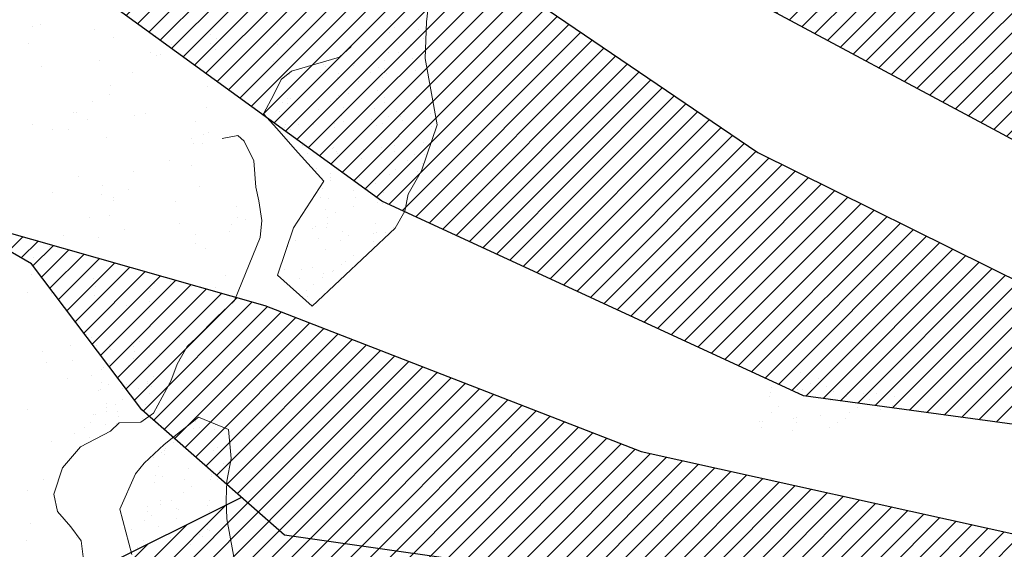
# Model space of a CAD drawing. Units: inches. Extents: x 1986 to 21484, y -1816 to 2016.
# Tile 60 of 85: x 3651.42 to 3662.33, y 1883.64 to 1889.5. Entities that reach past the tile are written whole.
import ezdxf

# ---------------------------------------------------------------- set-up
doc = ezdxf.new("R2010")
doc.units = ezdxf.units.IN
doc.layers.add('L-PLNT', color=84, linetype='Continuous', lineweight=13)
doc.layers.add('vfolhas', color=114, linetype='Continuous', lineweight=5)
doc.layers.add('vfolha2', color=110, linetype='Continuous')
doc.layers.add('vfolhas2', color=102, linetype='Continuous')
pattern_1 = [(45, (-2446.5133113, 50.986076), (-0.004419417382, 0.004419417382), [])]

# ---------------------------------------------------------------- blocks, each defined once
blk = doc.blocks.new('arbusto_PB_verde_grande')
at = {"layer": 'vfolha2'}
h = blk.add_hatch(dxfattribs=at)
h.set_pattern_fill('ANSI31', color=256, scale=0.05, style=0)
h.set_pattern_definition(pattern_1)
h.paths.add_polyline_path([(0.02944, 0.35651), (0.00028, 0.09048), (0.02625, -0.03934), (0.047, 0.06233), (0.06189, 0.09731), (0.09372, 0.26573), (0.09955, 0.43473), (0.08789, 0.61313), (0.0645, 0.72266), (0.04988, 0.6851), (0.0236, 0.51294)])
h.paths.add_polyline_path([(0.30106, 0.43789), (0.14225, 0.24871), (0.26685, 0.30022)])
h.paths.add_polyline_path([(0.37995, 0.22817), (0.23697, 0.15193), (0.18428, 0.09364), (0.11122, 0.04358), (0.02625, -0.03934), (0.28061, 0.04667), (0.36829, 0.07798), (0.46756, 0.11239), (0.61068, 0.19376), (0.71585, 0.27823), (0.55813, 0.25948)])
h.paths.add_polyline_path([(0.56101, -0.29441), (0.72752, -0.32573), (0.59024, -0.2412), (0.42962, -0.15982), (0.02625, -0.03934), (0.14922, -0.14107), (0.18838, -0.16604), (0.41501, -0.24435)])
h.paths.add_polyline_path([(-0.27429, -0.44776), (-0.30352, -0.72628), (-0.23923, -0.64175), (-0.15457, -0.45716), (0.02625, -0.03934), (-0.16328, -0.25376)])
h.paths.add_polyline_path([(-0.51963, -0.24744), (-0.67736, -0.32573), (-0.59558, -0.35072), (-0.40574, -0.32882), (-0.21007, -0.20995), (0.02625, -0.03934), (-0.14874, -0.06595), (-0.31518, -0.09101), (-0.41452, -0.15048)])
h.paths.add_polyline_path([(-0.52546, 0.25007), (-0.70947, 0.24698), (-0.51963, 0.1093), (-0.32979, 0.02167), (-0.07567, -0.0128), (-0.04234, -0.02148), (-0.35024, 0.1312)])
at = {"layer": 'vfolhas'}
h = blk.add_hatch(dxfattribs=at)
h.set_pattern_fill('ANSI31', color=256, scale=0.05, style=0)
h.set_pattern_definition(pattern_1)
h.paths.add_polyline_path([(-0.07279, 0.50669), (-0.18085, 0.65063), (-0.2334, 0.67253), (-0.20712, 0.53176), (-0.10785, 0.25007), (0.02625, -0.03934), (0.00028, 0.09048), (0.00816, 0.16241), (-0.04939, 0.29079)])
h.paths.add_polyline_path([(0.09902, 0.41929), (0.09372, 0.26573), (0.07906, 0.18814), (0.15506, 0.36901), (0.26606, 0.5505), (0.28356, 0.63504), (0.2485, 0.68819), (0.25145, 0.63504), (0.20178, 0.54426)])
h.paths.add_polyline_path([(0.12295, 0.24073), (0.047, 0.06233), (0.02625, -0.03934), (0.11122, 0.04358), (0.18428, 0.09364), (0.27478, 0.19376), (0.3215, 0.25323), (0.44129, 0.38467), (0.47634, 0.57866), (0.41789, 0.45347), (0.28939, 0.30954)])
h.paths.add_polyline_path([(0.58145, -0.03779), (0.70707, 0.01536), (0.78591, 0.04667), (0.74796, 0.06549), (0.62818, 0.08423), (0.52595, 0.09048), (0.39745, 0.04358), (0.02625, -0.03934), (0.25728, -0.03154), (0.43834, -0.0347)])
h.paths.add_polyline_path([(0.52022, -0.03647), (0.43834, -0.0347), (0.25728, -0.03154), (0.02625, -0.03934), (0.17964, -0.08515), (0.53768, -0.13167), (0.69541, -0.15357), (0.78591, -0.07852), (0.70413, -0.10042)])
h.paths.add_polyline_path([(0.27189, -0.21929), (0.14922, -0.14107), (0.02625, -0.03934), (0.15794, -0.31007), (0.29522, -0.42585), (0.41789, -0.49157), (0.56396, -0.56669), (0.5114, -0.48532), (0.39456, -0.34139)])
h.paths.add_polyline_path([(-0.05818, -0.47591), (-0.02312, -0.61984), (0.047, -0.80134), (0.08494, -0.59794), (0.07911, -0.4071), (0.03527, -0.25376), (0.02625, -0.03934), (-0.03773, -0.26001)])
h.paths.add_polyline_path([(-0.24218, 0.14054), (-0.11073, 0.06858), (0.02625, -0.03934), (-0.04235, 0.10871), (-0.21007, 0.23757), (-0.36485, 0.33145), (-0.47874, 0.40341), (-0.54303, 0.46288), (-0.49041, 0.33145), (-0.39408, 0.22192)])
h = blk.add_hatch(dxfattribs=at)
h.set_pattern_fill('ANSI31', color=256, scale=0.05, style=0)
h.set_pattern_definition(pattern_1)
h.paths.add_polyline_path([(-0.57219, 0.06233), (-0.7153, 0.10298), (-0.67736, 0.08107), (-0.62769, 0.01536), (-0.56347, -0.04095), (-0.26461, -0.0834), (-0.14874, -0.06595), (-0.10151, -0.05877), (-0.20418, -0.0472), (-0.40279, -0.00339)])
h.paths.add_polyline_path([(-0.56347, -0.04095), (-0.58279, -0.02401), (-0.72992, -0.09726), (-0.4334, -0.1679), (-0.41452, -0.15048), (-0.31518, -0.09101), (-0.26461, -0.0834)])
h.paths.add_polyline_path([(-0.2769, -0.47267), (-0.27429, -0.44776), (-0.16328, -0.25376), (0.02625, -0.03934), (-0.21007, -0.20995), (-0.2672, -0.24466), (-0.36485, -0.35697), (-0.42907, -0.46341), (-0.47586, -0.60425), (-0.37946, -0.57603)])
at = {"layer": 'vfolha2'}
for p, q in [((-0.52546, 0.25007), (-0.35024, 0.1312)), ((-0.51963, 0.1093), (-0.70947, 0.24698)), ((-0.35024, 0.1312), (-0.04234, -0.02148)), ((-0.32979, 0.02167), (-0.51963, 0.1093)), ((-0.07567, -0.0128), (-0.32979, 0.02167))]:
    blk.add_line(p, q, dxfattribs=at)
at = {"layer": 'vfolhas2'}
for p, q in [((-0.39408, 0.22192), (-0.24218, 0.14054)), ((-0.24218, 0.14054), (-0.11073, 0.06858)), ((-0.67736, 0.08107), (-0.7153, 0.10298)), ((-0.7153, 0.10298), (-0.57219, 0.06233)), ((-0.62769, 0.01536), (-0.67736, 0.08107)), ((-0.57219, 0.06233), (-0.40279, -0.00339)), ((-0.56347, -0.04095), (-0.62769, 0.01536)), ((-0.40279, -0.00339), (-0.20418, -0.0472)), ((-0.58279, -0.02401), (-0.72992, -0.09726)), ((-0.26461, -0.0834), (-0.56347, -0.04095))]:
    blk.add_line(p, q, dxfattribs=at)
blk = doc.blocks.new('PLANT-SHRUB')
for p, q in [((2168.859, 1883.625), (2168.859, 1883.625)), ((2168.775, 1883.571), (2168.775, 1883.571)), ((2168.989, 1883.571), (2168.989, 1883.571)), ((2168.895, 1883.414), (2168.895, 1883.414)), ((2168.999, 1883.4), (2168.999, 1883.4)), ((2169.001, 1883.318), (2169.001, 1883.318)), ((2169.162, 1883.379), (2169.162, 1883.379)), ((2169.258, 1883.364), (2169.258, 1883.364)), ((2169.335, 1883.373), (2169.335, 1883.373)), ((2169.433, 1883.343), (2169.433, 1883.343)), ((2169.537, 1883.329), (2169.537, 1883.329)), ((2169.124, 1883.18), (2169.124, 1883.18)), ((2169.161, 1883.213), (2169.161, 1883.213)), ((2169.236, 1883.069), (2169.236, 1883.069)), ((2169.32, 1883.123), (2169.32, 1883.123)), ((2169.516, 1883.166), (2169.516, 1883.166)), ((2169.858, 1883.068), (2169.858, 1883.068)), ((2169.246, 1882.979), (2169.246, 1882.979)), ((2169.725, 1883.004), (2169.725, 1883.004)), ((2169.757, 1882.981), (2169.757, 1882.981)), ((2169.762, 1883.038), (2169.762, 1883.038)), ((2169.249, 1882.85), (2169.249, 1882.85)), ((2169.353, 1882.836), (2169.353, 1882.836)), ((2169.462, 1882.816), (2169.462, 1882.816)), ((2169.504, 1882.781), (2169.504, 1882.781)), ((2169.516, 1882.815), (2169.516, 1882.815)), ((2169.526, 1882.822), (2169.526, 1882.822)), ((2169.787, 1882.779), (2169.787, 1882.779)), ((2169.891, 1882.765), (2169.891, 1882.765)), ((2170.027, 1882.775), (2170.027, 1882.775)), ((2170.053, 1882.744), (2170.053, 1882.744)), ((2170.084, 1882.815), (2170.084, 1882.815)), ((2169.352, 1882.663), (2169.352, 1882.663)), ((2169.697, 1882.568), (2169.697, 1882.568)), ((2169.744, 1882.596), (2169.744, 1882.596)), ((2169.781, 1882.622), (2169.781, 1882.622)), ((2175.39, 1879.961), (2175.094, 1879.497)), ((2175.094, 1879.497), (2174.956, 1879.339)), ((2175.321, 1879.464), (2175.321, 1879.464)), ((2175.295, 1879.398), (2175.295, 1879.398)), ((2175.332, 1879.432), (2175.332, 1879.432)), ((2175.425, 1879.45), (2175.425, 1879.45)), ((2175.429, 1879.419), (2175.429, 1879.419)), ((2175.587, 1879.428), (2175.587, 1879.428)), ((2174.956, 1879.339), (2174.808, 1879.191)), ((2175.178, 1879.301), (2175.178, 1879.301)), ((2174.808, 1879.191), (2174.601, 1879.043)), ((2175.097, 1879.216), (2175.097, 1879.216)), ((2175.147, 1879.241), (2175.147, 1879.241)), ((2175.686, 1879.221), (2175.686, 1879.221)), ((2174.601, 1879.043), (2174.403, 1878.787)), ((2174.703, 1879.028), (2174.703, 1879.028)), ((2174.79, 1879.054), (2174.79, 1879.054)), ((2174.874, 1879.107), (2174.874, 1879.107)), ((2174.893, 1879.04), (2174.893, 1879.04)), ((2174.923, 1879.057), (2174.923, 1879.057)), ((2175.413, 1879.053), (2175.413, 1879.053)), ((2175.416, 1879.034), (2175.416, 1879.034)), ((2175.497, 1879.106), (2175.497, 1879.106)), ((2175.697, 1879.041), (2175.697, 1879.041)), ((2175.884, 1878.61), (2176.131, 1879.063)), ((2175.927, 1879.036), (2175.927, 1879.036)), ((2176.035, 1879.051), (2176.035, 1879.051)), ((2174.865, 1879.006), (2174.865, 1879.006)), ((2174.886, 1879.023), (2174.886, 1879.023)), ((2175.136, 1878.97), (2175.136, 1878.97)), ((2175.24, 1878.957), (2175.24, 1878.957)), ((2175.403, 1878.935), (2175.403, 1878.935)), ((2174.623, 1878.853), (2174.623, 1878.853)), ((2174.687, 1878.841), (2174.687, 1878.841)), ((2175.134, 1878.855), (2175.134, 1878.855)), ((2175.487, 1878.848), (2175.487, 1878.848)), ((2175.523, 1878.881), (2175.523, 1878.881)), ((2175.674, 1878.9), (2175.674, 1878.9)), ((2175.674, 1878.836), (2175.674, 1878.836)), ((2175.778, 1878.886), (2175.778, 1878.886)), ((2175.941, 1878.864), (2175.941, 1878.864)), ((2174.403, 1878.787), (2174.552, 1878.462)), ((2175.016, 1878.8), (2175.016, 1878.8)), ((2175.639, 1878.799), (2175.639, 1878.799)), ((2176.561, 1878.739), (2176.437, 1878.57)), ((2174.476, 1878.648), (2174.476, 1878.648)), ((2174.513, 1878.681), (2174.513, 1878.681)), ((2174.713, 1878.607), (2174.713, 1878.607)), ((2174.88, 1878.655), (2174.88, 1878.655)), ((2175.288, 1878.665), (2175.288, 1878.665)), ((2175.335, 1878.606), (2175.335, 1878.606)), ((2175.403, 1878.649), (2175.403, 1878.649)), ((2175.489, 1878.442), (2175.884, 1878.61)), ((2174.629, 1878.553), (2174.629, 1878.553)), ((2174.681, 1878.513), (2174.681, 1878.513)), ((2175.114, 1878.506), (2175.114, 1878.506)), ((2175.251, 1878.552), (2175.251, 1878.552)), ((2176.437, 1878.57), (2176.415, 1878.379)), ((2176.454, 1878.508), (2176.454, 1878.508)), ((2171.325, 1878.363), (2171.534, 1878.429)), ((2171.534, 1878.429), (2172.793, 1878.429)), ((2171.541, 1878.409), (2171.541, 1878.409)), ((2171.645, 1878.395), (2171.645, 1878.395)), ((2171.807, 1878.374), (2171.807, 1878.374)), ((2171.855, 1878.423), (2171.855, 1878.423)), ((2172.793, 1878.429), (2172.84, 1877.916)), ((2174.552, 1878.462), (2175.035, 1878.422)), ((2174.61, 1878.468), (2174.61, 1878.468)), ((2174.952, 1878.477), (2174.952, 1878.477)), ((2175.035, 1878.422), (2175.341, 1878.422)), ((2175.056, 1878.464), (2175.056, 1878.464)), ((2175.077, 1878.472), (2175.077, 1878.472)), ((2175.121, 1878.47), (2175.121, 1878.47)), ((2175.219, 1878.442), (2175.219, 1878.442)), ((2175.341, 1878.422), (2175.489, 1878.442)), ((2176.415, 1878.379), (2176.404, 1878.154)), ((2171.171, 1878.253), (2171.325, 1878.363)), ((2171.72, 1878.318), (2171.72, 1878.318)), ((2171.743, 1878.306), (2171.743, 1878.306)), ((2172.078, 1878.338), (2172.078, 1878.338)), ((2172.182, 1878.324), (2172.182, 1878.324)), ((2172.243, 1878.311), (2172.243, 1878.311)), ((2172.345, 1878.303), (2172.345, 1878.303)), ((2172.366, 1878.304), (2172.366, 1878.304)), ((2172.492, 1878.282), (2172.492, 1878.282)), ((2172.616, 1878.267), (2172.616, 1878.267)), ((2172.754, 1878.313), (2172.754, 1878.313)), ((2170.412, 1877.913), (2170.885, 1878.166)), ((2170.885, 1878.166), (2171.171, 1878.253)), ((2171.656, 1878.241), (2171.656, 1878.241)), ((2172.456, 1878.248), (2172.456, 1878.248)), ((2172.72, 1878.254), (2172.72, 1878.254)), ((2176.404, 1878.154), (2176.302, 1877.986)), ((2176.442, 1878.247), (2176.442, 1878.247)), ((2176.879, 1878.156), (2176.879, 1878.156)), ((2170.734, 1878.06), (2170.734, 1878.06)), ((2170.818, 1878.113), (2170.818, 1878.113)), ((2170.926, 1878.137), (2170.926, 1878.137)), ((2171.356, 1878.059), (2171.356, 1878.059)), ((2171.44, 1878.112), (2171.44, 1878.112)), ((2171.445, 1878.048), (2171.445, 1878.048)), ((2171.45, 1878.13), (2171.45, 1878.13)), ((2171.482, 1878.082), (2171.482, 1878.082)), ((2171.961, 1878.133), (2171.961, 1878.133)), ((2171.978, 1878.057), (2171.978, 1878.057)), ((2172.062, 1878.111), (2172.062, 1878.111)), ((2172.257, 1878.066), (2172.257, 1878.066)), ((2172.5, 1878.113), (2172.5, 1878.113)), ((2172.6, 1878.056), (2172.6, 1878.056)), ((2172.685, 1878.11), (2172.685, 1878.11)), ((2174.885, 1878.087), (2174.503, 1877.963)), ((2175.054, 1878.065), (2174.885, 1878.087)), ((2175.011, 1878.05), (2175.011, 1878.05)), ((2175.054, 1878.065), (2175.054, 1878.065)), ((2175.234, 1877.907), (2175.054, 1878.065)), ((2176.711, 1878.048), (2176.711, 1878.048)), ((2170.656, 1877.95), (2170.656, 1877.95)), ((2170.818, 1877.987), (2170.818, 1877.987)), ((2170.922, 1877.973), (2170.922, 1877.973)), ((2171.085, 1877.952), (2171.085, 1877.952)), ((2171.167, 1877.952), (2171.167, 1877.952)), ((2174.503, 1877.963), (2174.323, 1877.874)), ((2174.543, 1877.967), (2174.543, 1877.967)), ((2174.88, 1877.956), (2174.88, 1877.956)), ((2174.961, 1877.962), (2174.961, 1877.962)), ((2176.302, 1877.986), (2176.033, 1877.84)), ((2170.005, 1877.287), (2170.412, 1877.913)), ((2170.435, 1877.848), (2170.435, 1877.848)), ((2170.472, 1877.882), (2170.472, 1877.882)), ((2171.246, 1877.866), (2171.246, 1877.866)), ((2171.356, 1877.916), (2171.356, 1877.916)), ((2171.46, 1877.902), (2171.46, 1877.902)), ((2171.623, 1877.881), (2171.623, 1877.881)), ((2171.707, 1877.933), (2171.707, 1877.933)), ((2171.894, 1877.845), (2171.894, 1877.845)), ((2171.998, 1877.831), (2171.998, 1877.831)), ((2172.046, 1877.872), (2172.046, 1877.872)), ((2172.083, 1877.906), (2172.083, 1877.906)), ((2172.23, 1877.926), (2172.23, 1877.926)), ((2172.84, 1877.916), (2172.352, 1877.656)), ((2172.741, 1877.928), (2172.741, 1877.928)), ((2172.84, 1877.916), (2172.84, 1877.916)), ((2174.323, 1877.874), (2174.109, 1877.806)), ((2174.26, 1877.844), (2174.26, 1877.844)), ((2174.323, 1877.874), (2174.323, 1877.874)), ((2174.39, 1877.827), (2174.39, 1877.827)), ((2174.701, 1877.852), (2174.701, 1877.852)), ((2174.741, 1877.829), (2174.741, 1877.829)), ((2174.768, 1877.895), (2174.768, 1877.895)), ((2175.199, 1877.851), (2175.199, 1877.851)), ((2175.369, 1877.907), (2175.234, 1877.907)), ((2175.266, 1877.894), (2175.266, 1877.894)), ((2175.729, 1877.806), (2175.369, 1877.907)), ((2176.033, 1877.84), (2175.729, 1877.806)), ((2170.374, 1877.771), (2170.374, 1877.771)), ((2170.914, 1877.752), (2170.914, 1877.752)), ((2170.96, 1877.806), (2170.96, 1877.806)), ((2171.437, 1877.745), (2171.437, 1877.745)), ((2171.582, 1877.805), (2171.582, 1877.805)), ((2171.948, 1877.748), (2171.948, 1877.748)), ((2172.161, 1877.81), (2172.161, 1877.81)), ((2172.204, 1877.804), (2172.204, 1877.804)), ((2172.432, 1877.774), (2172.432, 1877.774)), ((2172.536, 1877.761), (2172.536, 1877.761)), ((2173.378, 1877.795), (2172.693, 1877.482)), ((2173.378, 1877.795), (2173.378, 1877.795)), ((2173.648, 1877.795), (2173.378, 1877.795)), ((2173.974, 1877.806), (2173.648, 1877.795)), ((2174.109, 1877.806), (2173.974, 1877.806)), ((2174.071, 1877.796), (2174.071, 1877.796)), ((2174.327, 1877.817), (2174.327, 1877.817)), ((2174.607, 1877.798), (2174.607, 1877.798)), ((2174.691, 1877.787), (2174.691, 1877.787)), ((2174.711, 1877.802), (2174.711, 1877.802)), ((2174.736, 1877.819), (2174.736, 1877.819)), ((2174.821, 1877.77), (2174.821, 1877.77)), ((2175.038, 1877.742), (2175.038, 1877.742)), ((2175.121, 1877.731), (2175.121, 1877.731)), ((2175.168, 1877.804), (2175.168, 1877.804)), ((2175.36, 1877.816), (2175.36, 1877.816)), ((2175.586, 1877.798), (2175.586, 1877.798)), ((2176.278, 1877.785), (2176.278, 1877.785)), ((2176.486, 1877.758), (2176.486, 1877.758)), ((2170.656, 1877.613), (2170.656, 1877.613)), ((2171.036, 1877.673), (2171.036, 1877.673)), ((2171.073, 1877.706), (2171.073, 1877.706)), ((2171.279, 1877.612), (2171.279, 1877.612)), ((2172.352, 1877.656), (2171.755, 1877.508)), ((2171.847, 1877.69), (2171.847, 1877.69)), ((2171.901, 1877.611), (2171.901, 1877.611)), ((2174.101, 1877.675), (2174.101, 1877.675)), ((2174.384, 1877.65), (2174.384, 1877.65)), ((2174.533, 1877.659), (2174.533, 1877.659)), ((2174.552, 1877.656), (2174.552, 1877.656)), ((2174.882, 1877.65), (2174.882, 1877.65)), ((2174.951, 1877.654), (2174.951, 1877.654)), ((2175.192, 1877.661), (2175.192, 1877.661)), ((2175.221, 1877.688), (2175.221, 1877.688)), ((2175.251, 1877.714), (2175.251, 1877.714)), ((2175.36, 1877.656), (2175.36, 1877.656)), ((2175.38, 1877.649), (2175.38, 1877.649)), ((2175.468, 1877.685), (2175.468, 1877.685)), ((2175.551, 1877.674), (2175.551, 1877.674)), ((2175.681, 1877.657), (2175.681, 1877.657)), ((2170.2, 1877.551), (2170.2, 1877.551)), ((2170.363, 1877.529), (2170.363, 1877.529)), ((2170.572, 1877.559), (2170.572, 1877.559)), ((2170.644, 1877.565), (2170.644, 1877.565)), ((2171.155, 1877.567), (2171.155, 1877.567)), ((2171.194, 1877.558), (2171.194, 1877.558)), ((2171.673, 1877.531), (2171.673, 1877.531)), ((2171.695, 1877.548), (2171.695, 1877.548)), ((2171.755, 1877.508), (2171.743, 1877.034)), ((2171.817, 1877.557), (2171.817, 1877.557)), ((2173.269, 1877.524), (2173.269, 1877.524)), ((2173.429, 1877.548), (2173.429, 1877.548)), ((2174.317, 1877.509), (2174.317, 1877.509)), ((2174.383, 1877.501), (2174.383, 1877.501)), ((2174.413, 1877.528), (2174.413, 1877.528)), ((2174.726, 1877.511), (2174.726, 1877.511)), ((2175.033, 1877.515), (2175.033, 1877.515)), ((2175.919, 1877.544), (2175.919, 1877.544)), ((2170.634, 1877.494), (2170.634, 1877.494)), ((2170.738, 1877.48), (2170.738, 1877.48)), ((2170.837, 1877.49), (2170.837, 1877.49)), ((2170.901, 1877.458), (2170.901, 1877.458)), ((2171.172, 1877.423), (2171.172, 1877.423)), ((2171.276, 1877.409), (2171.276, 1877.409)), ((2171.636, 1877.497), (2171.636, 1877.497)), ((2172.693, 1877.482), (2172.551, 1877.356)), ((2174.46, 1877.404), (2174.46, 1877.404)), ((2174.543, 1877.393), (2174.543, 1877.393)), ((2174.572, 1877.452), (2174.572, 1877.452)), ((2174.639, 1877.495), (2174.639, 1877.495)), ((2175.07, 1877.451), (2175.07, 1877.451)), ((2175.137, 1877.494), (2175.137, 1877.494)), ((2175.157, 1877.495), (2175.157, 1877.495)), ((2169.719, 1877.001), (2170.005, 1877.287)), ((2170.176, 1877.307), (2170.176, 1877.307)), ((2170.362, 1877.386), (2170.362, 1877.386)), ((2170.626, 1877.297), (2170.626, 1877.297)), ((2170.663, 1877.331), (2170.663, 1877.331)), ((2170.798, 1877.306), (2170.798, 1877.306)), ((2170.901, 1877.367), (2170.901, 1877.367)), ((2171.421, 1877.305), (2171.421, 1877.305)), ((2171.424, 1877.36), (2171.424, 1877.36)), ((2171.438, 1877.388), (2171.438, 1877.388)), ((2171.438, 1877.315), (2171.438, 1877.315)), ((2171.71, 1877.352), (2171.71, 1877.352)), ((2172.551, 1877.356), (2172.425, 1877.174)), ((2173.614, 1877.357), (2173.614, 1877.357)), ((2174.523, 1877.351), (2174.523, 1877.351)), ((2174.673, 1877.376), (2174.673, 1877.376)), ((2174.864, 1877.361), (2174.864, 1877.361)), ((2174.89, 1877.347), (2174.89, 1877.347)), ((2174.894, 1877.388), (2174.894, 1877.388)), ((2174.941, 1877.346), (2174.941, 1877.346)), ((2174.974, 1877.336), (2174.974, 1877.336)), ((2175.104, 1877.319), (2175.104, 1877.319)), ((2170.108, 1877.186), (2170.108, 1877.186)), ((2170.631, 1877.179), (2170.631, 1877.179)), ((2171.142, 1877.182), (2171.142, 1877.182)), ((2172.425, 1877.174), (2172.346, 1877.04)), ((2172.682, 1877.224), (2172.682, 1877.224)), ((2172.89, 1877.197), (2172.89, 1877.197)), ((2174.705, 1877.215), (2174.705, 1877.215)), ((2174.716, 1877.203), (2174.716, 1877.203)), ((2174.753, 1877.249), (2174.753, 1877.249)), ((2169.873, 1877.114), (2169.873, 1877.114)), ((2169.912, 1877.071), (2169.912, 1877.071)), ((2170.427, 1877.115), (2170.427, 1877.115)), ((2170.495, 1877.113), (2170.495, 1877.113)), ((2171.117, 1877.111), (2171.117, 1877.111)), ((2171.227, 1877.122), (2171.227, 1877.122)), ((2171.264, 1877.156), (2171.264, 1877.156)), ((2171.682, 1877.162), (2171.682, 1877.162)), ((2171.74, 1877.11), (2171.74, 1877.11)), ((2172.728, 1877.149), (2172.728, 1877.149)), ((2172.823, 1877.162), (2172.823, 1877.162)), ((2173.215, 1877.154), (2173.215, 1877.154)), ((2173.751, 1877.154), (2173.751, 1877.154)), ((2173.758, 1877.082), (2173.758, 1877.082)), ((2174.067, 1877.159), (2174.067, 1877.159)), ((2174.83, 1877.115), (2174.83, 1877.115)), ((2175.312, 1877.157), (2175.312, 1877.157)), ((2175.876, 1877.102), (2175.876, 1877.102)), ((2169.522, 1876.836), (2169.719, 1877.001)), ((2169.788, 1877.06), (2169.788, 1877.06)), ((2169.838, 1876.999), (2169.838, 1876.999)), ((2170.016, 1877.057), (2170.016, 1877.057)), ((2170.178, 1877.036), (2170.178, 1877.036)), ((2170.253, 1876.956), (2170.253, 1876.956)), ((2170.349, 1877.001), (2170.349, 1877.001)), ((2170.411, 1877.059), (2170.411, 1877.059)), ((2170.45, 1877), (2170.45, 1877)), ((2170.554, 1876.987), (2170.554, 1876.987)), ((2170.716, 1876.965), (2170.716, 1876.965)), ((2170.889, 1876.982), (2170.889, 1876.982)), ((2171.033, 1877.058), (2171.033, 1877.058)), ((2171.412, 1876.975), (2171.412, 1876.975)), ((2171.655, 1877.057), (2171.655, 1877.057)), ((2171.743, 1877.034), (2171.732, 1876.726)), ((2172.346, 1877.04), (2172.164, 1876.811)), ((2172.654, 1877.054), (2172.654, 1877.054)), ((2173.193, 1876.971), (2173.193, 1876.971)), ((2173.267, 1877.039), (2173.267, 1877.039)), ((2173.899, 1877.052), (2173.899, 1877.052)), ((2173.966, 1877.055), (2173.966, 1877.055)), ((2174.291, 1877.012), (2174.291, 1877.012)), ((2174.816, 1877.006), (2174.816, 1877.006)), ((2175.143, 1877.05), (2175.143, 1877.05)), ((2170.217, 1876.922), (2170.217, 1876.922)), ((2170.988, 1876.93), (2170.988, 1876.93)), ((2171.028, 1876.94), (2171.028, 1876.94)), ((2171.092, 1876.916), (2171.092, 1876.916)), ((2171.254, 1876.894), (2171.254, 1876.894)), ((2171.526, 1876.859), (2171.526, 1876.859)), ((2171.63, 1876.845), (2171.63, 1876.845)), ((2174.833, 1876.941), (2174.833, 1876.941)), ((2175.041, 1876.913), (2175.041, 1876.913)), ((2175.366, 1876.871), (2175.366, 1876.871)), ((2170.015, 1876.807), (2170.015, 1876.807)), ((2170.018, 1876.74), (2170.018, 1876.74)), ((2170.095, 1876.801), (2170.095, 1876.801)), ((2170.618, 1876.794), (2170.618, 1876.794)), ((2170.637, 1876.805), (2170.637, 1876.805)), ((2170.817, 1876.747), (2170.817, 1876.747)), ((2170.854, 1876.78), (2170.854, 1876.78)), ((2171.13, 1876.797), (2171.13, 1876.797)), ((2171.259, 1876.804), (2171.259, 1876.804)), ((2171.629, 1876.764), (2171.629, 1876.764)), ((2171.669, 1876.777), (2171.669, 1876.777)), ((2172.164, 1876.811), (2172.093, 1876.582)), ((2173.243, 1876.754), (2173.243, 1876.754)), ((2174.29, 1876.74), (2174.29, 1876.74)), ((2175.312, 1876.745), (2175.312, 1876.745)), ((2170.687, 1876.628), (2170.511, 1876.628)), ((2171.182, 1876.375), (2170.687, 1876.628)), ((2171.732, 1876.726), (2171.732, 1876.507)), ((2174.468, 1876.688), (2174.468, 1876.688)), ((2170.872, 1876.557), (2170.872, 1876.557)), ((2170.876, 1876.597), (2170.876, 1876.597)), ((2170.956, 1876.611), (2170.956, 1876.611)), ((2171.399, 1876.59), (2171.399, 1876.59)), ((2171.418, 1876.571), (2171.418, 1876.571)), ((2171.455, 1876.605), (2171.455, 1876.605)), ((2171.494, 1876.556), (2171.494, 1876.556)), ((2171.578, 1876.61), (2171.578, 1876.61)), ((2172.093, 1876.582), (2172.101, 1876.487)), ((2172.795, 1876.606), (2172.795, 1876.606)), ((2173.107, 1876.547), (2173.107, 1876.547)), ((2174.351, 1876.545), (2174.351, 1876.545)), ((2174.394, 1876.62), (2174.394, 1876.62)), ((2171.117, 1876.412), (2171.117, 1876.412)), ((2171.501, 1876.43), (2171.325, 1876.364)), ((2171.732, 1876.507), (2171.501, 1876.43)), ((2172.101, 1876.487), (2172.251, 1876.392)), ((2171.325, 1876.364), (2171.182, 1876.375)), ((2171.219, 1876.389), (2171.219, 1876.389)), ((2172.703, 1876.379), (2172.703, 1876.379)), ((2173.725, 1876.384), (2173.725, 1876.384)), ((2174.805, 1876.345), (2174.805, 1876.345)), ((2172.313, 1876.238), (2172.313, 1876.238)), ((2172.374, 1876.22), (2172.374, 1876.22)), ((2172.447, 1876.288), (2172.447, 1876.288)), ((2172.521, 1876.21), (2172.521, 1876.21)), ((2173.997, 1876.256), (2173.997, 1876.256)), ((2171.255, 1876.163), (2171.255, 1876.163)), ((2172.5, 1876.161), (2172.5, 1876.161)), ((2172.846, 1876.167), (2172.846, 1876.167)), ((2173.389, 1876.096), (2173.389, 1876.096)), ((2173.745, 1876.159), (2173.745, 1876.159)), ((2174.989, 1876.156), (2174.989, 1876.156)), ((2171.087, 1876.056), (2171.087, 1876.056)), ((2171.116, 1876.018), (2171.116, 1876.018)), ((2172.139, 1876.023), (2172.139, 1876.023)), ((2172.331, 1876.054), (2172.331, 1876.054)), ((2173.218, 1875.984), (2173.218, 1875.984)), ((2173.576, 1876.051), (2173.576, 1876.051)), ((2173.597, 1876.069), (2173.597, 1876.069)), ((2173.922, 1876.026), (2173.922, 1876.026)), ((2174.821, 1876.049), (2174.821, 1876.049)), ((2173.575, 1875.87), (2173.575, 1875.87)), ((2173.649, 1875.937), (2173.649, 1875.937)), ((2174.264, 1875.97), (2174.264, 1875.97)), ((2174.465, 1875.954), (2174.465, 1875.954)), ((2174.673, 1875.927), (2174.673, 1875.927)), ((2171.976, 1875.856), (2171.976, 1875.856)), ((2171.539, 1875.549), (2171.539, 1875.549)), ((2171.628, 1875.537), (2171.628, 1875.537)), ((2171.632, 1875.622), (2171.632, 1875.622)), ((2172.678, 1875.609), (2172.678, 1875.609)), ((2172.784, 1875.547), (2172.784, 1875.547)), ((2173.7, 1875.614), (2173.7, 1875.614)), ((2174.029, 1875.544), (2174.029, 1875.544)), ((2171.555, 1875.47), (2171.555, 1875.47)), ((2173.177, 1875.505), (2173.177, 1875.505)), ((2171.945, 1875.251), (2171.945, 1875.251)), ((2172.114, 1875.252), (2172.114, 1875.252)), ((2172.153, 1875.224), (2172.153, 1875.224)), ((2173.193, 1875.214), (2173.193, 1875.214)), ((2172.177, 1875.16), (2172.177, 1875.16)), ((2172.478, 1875.181), (2172.478, 1875.181)), ((2172.756, 1875.119), (2172.756, 1875.119)), ((2172.83, 1875.186), (2172.83, 1875.186)), ((2173.021, 1875.11), (2173.021, 1875.11)), ((2173.422, 1875.158), (2173.422, 1875.158)), ((2172.009, 1875.053), (2172.009, 1875.053)), ((2173.229, 1875.082), (2173.229, 1875.082)), ((2173.253, 1875.05), (2173.253, 1875.05)), ((2173.554, 1875.04), (2173.554, 1875.04)), ((2172.653, 1874.839), (2172.653, 1874.839)), ((2173.675, 1874.844), (2173.675, 1874.844)), ((2172.358, 1874.754), (2172.358, 1874.754)), ((2172.461, 1874.546), (2172.461, 1874.546)), ((2173.168, 1874.443), (2173.168, 1874.443)), ((2173.099, 1874.157), (2173.099, 1874.157)), ((2172.86, 1874.096), (2172.86, 1874.096)), ((2172.93, 1874.05), (2172.93, 1874.05))]:
    blk.add_line(p, q)

msp = doc.modelspace()

# ---------------------------------------------------------------- block references
at = {"layer": 'L-PLNT', "rotation": 223.1883365522388}
msp.add_blockref('PLANT-SHRUB', (3953.27, 4742.965), dxfattribs=at)
at = {"layer": 'L-PLNT', "xscale": 24.60366729364114, "yscale": 24.60366729364114, "zscale": 24.60366729364114}
msp.add_blockref('arbusto_PB_verde_grande', (3668.218, 1884.805), dxfattribs=at)

doc.saveas('drawing.dxf')
